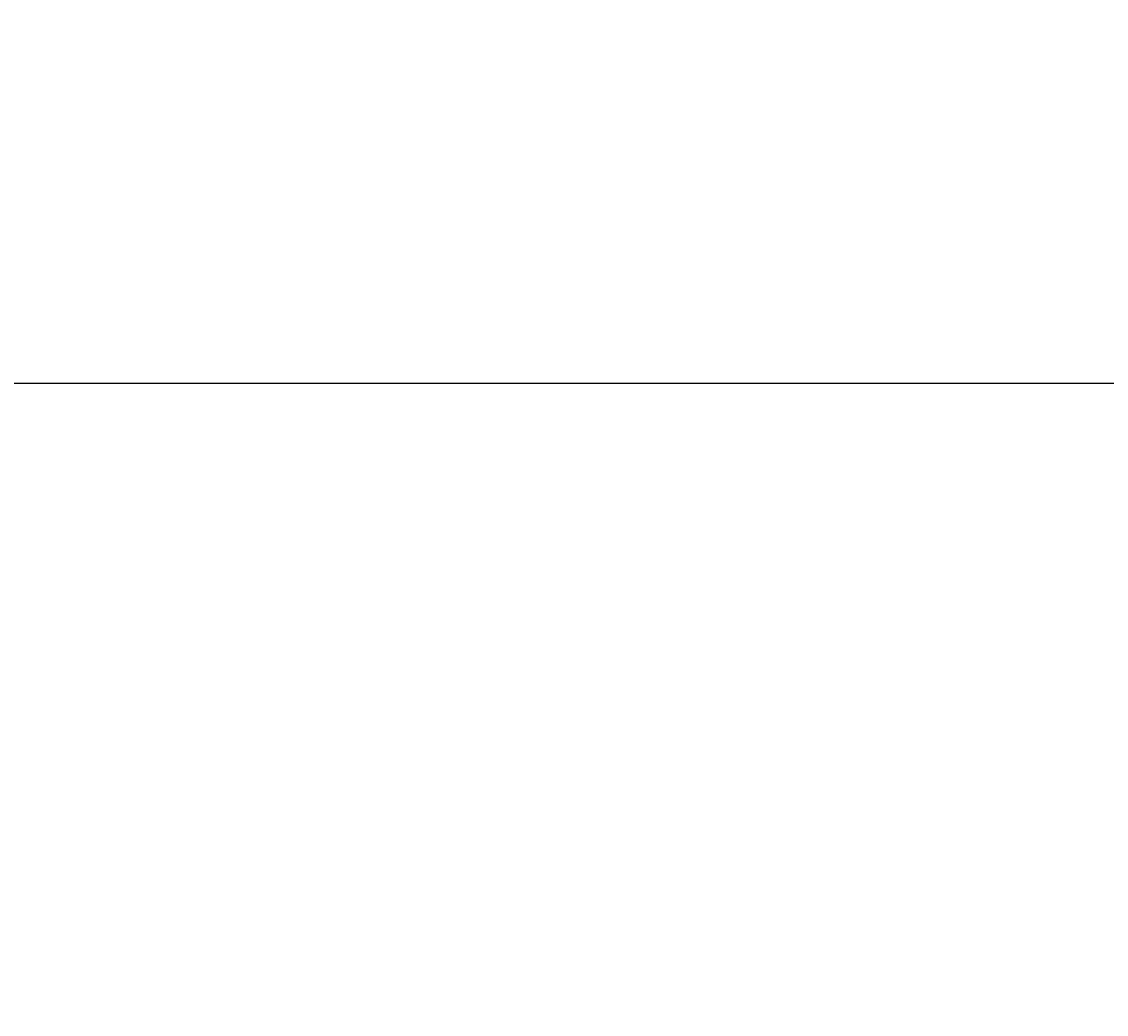
# Model space of a CAD drawing. Units: inches. Extents: x 182 to 1022, y -617 to 111.
# Tile 9 of 33: x 363 to 399, y -340 to -308. Entities that reach past the tile are written whole.
import ezdxf

# ---------------------------------------------------------------- set-up
doc = ezdxf.new("R2010")
doc.units = ezdxf.units.IN
doc.header["$MEASUREMENT"] = 0
doc.layers.add('A-ANNO-DIMS', color=2, linetype='Continuous', lineweight=18)
doc.styles.get("Standard").update_dxf_attribs({"font": 'arial.ttf'})
doc.dimstyles.get("Standard").update_dxf_attribs({"dimtxt": 0.18, "dimasz": 0.18, "dimexe": 0.18, "dimexo": 0.0625, "dimgap": 0.09, "dimtad": 0, "dimtih": 1, "dimtoh": 1, "dimdec": 1, "dimzin": 0, "dimdsep": 46, "dimlunit": 4, "dimtxsty": 'Standard', "dimcen": 0.09, "dimadec": 0, "dimazin": 0, "dimtfac": 1, "dimtdec": 1, "dimtofl": 0, "dimtmove": 0, "dimatfit": 3, "dimfxl": 1, "dimtolj": 1, "dimtzin": 0, "dimarcsym": 0})

# ---------------------------------------------------------------- blocks, each defined once
blk = doc.blocks.new('*D26')
at = {"layer": 'A-ANNO-DIMS', "color": 0, "lineweight": -2, "transparency": 16777216}
for p, q in [((257.848, -296.884), (257.848, -319.733)), ((409.388, -296.884), (409.388, -319.733)), ((258.028, -319.553), (331.642, -319.553)), ((409.208, -319.553), (335.594, -319.553))]:
    blk.add_line(p, q, dxfattribs=at)
at = {"layer": 'A-ANNO-DIMS', "color": 0, "transparency": 16777216}
for points in [[(258.028, -319.523), (258.028, -319.583), (257.848, -319.553)], [(409.208, -319.523), (409.208, -319.583), (409.388, -319.553)]]:
    blk.add_solid(points, dxfattribs=at)
at = {"layer": 'Defpoints', "color": 0, "transparency": 16777216}
for p in [(257.848, -296.822), (409.388, -296.822), (409.388, -319.553)]:
    blk.add_point(p, dxfattribs=at)
at = {"layer": 'A-ANNO-DIMS', "color": 0, "transparency": 16777216, "insert": (333.618, -319.553), "char_height": 0.18, "attachment_point": 5}
blk.add_mtext('\\A1;LOUNGE GROUP 12\'-7 1/2" TYP.', dxfattribs=at)
blk = doc.blocks.new('*D39')
at = {"layer": 'A-ANNO-DIMS', "color": 0, "lineweight": -2, "transparency": 16777216}
for p, q in [((238.398, -288.54), (1015.285, -288.54)), ((1015.105, -288.72), (1015.105, -346.775)), ((1015.105, -405.193), (1015.105, -347.138)), ((238.427, -405.373), (1015.285, -405.373))]:
    blk.add_line(p, q, dxfattribs=at)
at = {"layer": 'A-ANNO-DIMS', "color": 0, "transparency": 16777216}
for points in [[(1015.075, -288.72), (1015.135, -288.72), (1015.105, -288.54)], [(1015.075, -405.193), (1015.135, -405.193), (1015.105, -405.373)]]:
    blk.add_solid(points, dxfattribs=at)
at = {"layer": 'Defpoints', "color": 0, "transparency": 16777216}
for p in [(238.335, -288.54), (1015.105, -288.54), (238.364, -405.373)]:
    blk.add_point(p, dxfattribs=at)
at = {"layer": 'A-ANNO-DIMS', "color": 0, "transparency": 16777216, "insert": (1015.105, -346.956), "char_height": 0.18, "attachment_point": 5}
blk.add_mtext('\\A1;9\'-9"', dxfattribs=at)

msp = doc.modelspace()

# ---------------------------------------------------------------- dimensions: what is measured, and where the dimension line sits
at = {"layer": 'A-ANNO-DIMS'}
dim = msp.add_linear_dim(base=(1015.105, -288.54), p1=(238.364, -405.373), p2=(238.335, -288.54), angle=90, dimstyle='Standard', override={"dimdec": 1, "dimlfac": 1, "dimrnd": 0, "dimzin": 1, "dimdsep": 46, "dimlunit": 4, "dimfrac": 2}, dxfattribs=at)
dim.commit()
dim.dimension.update_dxf_attribs({"geometry": '*D39', "text_midpoint": (1015.105, -346.956)})
dim = msp.add_linear_dim(base=(409.388, -319.553), p1=(257.848, -296.822), p2=(409.388, -296.822), text='LOUNGE GROUP <> TYP.', dimstyle='Standard', override={"dimdec": 1, "dimlfac": 1, "dimrnd": 0, "dimzin": 1, "dimdsep": 46, "dimlunit": 4, "dimfrac": 2}, dxfattribs=at)
dim.commit()
dim.dimension.update_dxf_attribs({"geometry": '*D26', "text_midpoint": (333.618, -319.553)})

doc.saveas('drawing.dxf')
